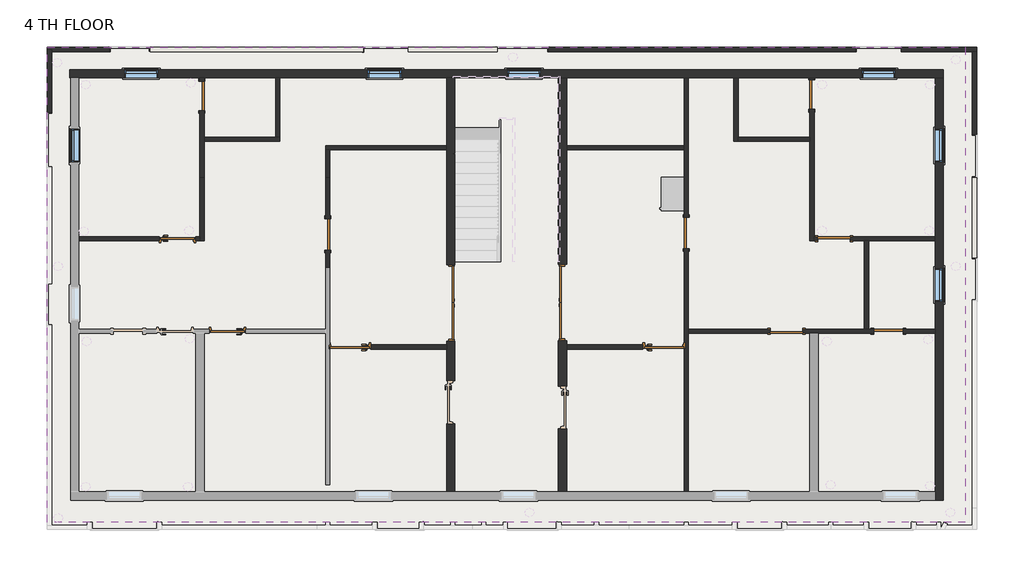
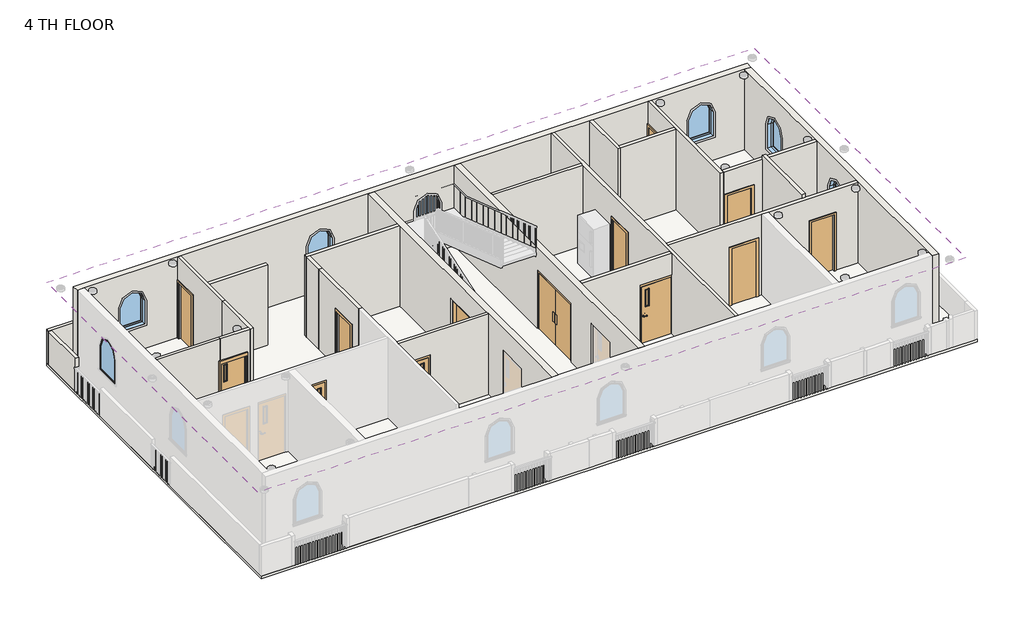
# One storey, part 2 of 7: 32 walls, 13 doors, 7 windows, 1 covering, 1 slab.
# Revit data of these elements (continued)
# Elements 6, 7 (IfcDoor, "Door-Passage-Single-Vision_Lite : 3'X7'") (continued)
#   Swing Angle = 90.00°
#   Rough Width = 3' - 4"
#   Rough Height = 7' - 4"
#   Masonry Inset = 0' - 1"
#   MFOpeningWidth = 0' - 4"
#   MFOpeningHeight = 0' - 4"
#   Inset Calculate = 0' - 4"
#   Masonry Frame = yes
#   Dry Wall Frame = no
#   Phase Created = New Construction
#   Materials on its faces: "Metal - Paint Finish - Grey", "Aluminum", "Wood - Birch", "Glass"
# Elements 8, 9 (IfcDoor, "Single-Flush : 2'10\" x 7'")
#   Phase Created = New Construction
#   Materials on its faces: "Door - Frame", "Door - Panel"
# Elements 10, 11 (IfcDoor, "Single-Flush : 2'11\"x 7'")
#   Phase Created = New Construction
#   Materials on its faces: "Door - Frame", "Door - Panel"
# Elements 12, 13, 14 (IfcDoor, "Single-Flush : 2'8\"x 7'")
#   Phase Created = New Construction
#   Materials on its faces: "Door - Frame", "Door - Panel"
# Element 15 (IfcSlab, "LW Concrete on Metal Deck")
#   Height Offset From Level = 0' - 0"
#   Phase Created = New Construction
#   Materials on its faces: "Metal Deck", "Concrete, Lightweight"
# Elements 16, 17, 18, 19, 20, 21, 22, 23, 24, 25, 26, 27, 28, 29, 31, 32, 33 (IfcWall, "Generic - 4.5\"")
#   Top Offset = -0' - 6"
#   Base Offset = 0' - 0"
#   wall height = 10' - 0"
#   Phase Created = New Construction
#   Base Constraint = 4 TH FLOOR
#   Top Constraint = 5TH FLOOR
#   Materials on its faces: "Default Wall"
# Elements 30, 40 (IfcWall, "Generic - 4.5\"")
#   Top Offset = -6' - 0"
#   Base Offset = 0' - 0"
#   wall height = 4' - 6"
#   Phase Created = New Construction
#   Base Constraint = 4 TH FLOOR
#   Top Constraint = 5TH FLOOR
#   Materials on its faces: "Default Wall"
# Element 34 (IfcWall, "Generic - 4.5\"")
#   Top Offset = -6' - 4.43284"
#   Base Offset = 0' - 0"
#   wall height = 4' - 1.56716"
#   Phase Created = New Construction
#   Base Constraint = 4 TH FLOOR
#   Top Constraint = 5TH FLOOR
#   Materials on its faces: "Default Wall"
# Element 35 (IfcWall, "Generic - 4.5\"")
#   Top Offset = -6' - 3.86561"
#   Base Offset = 0' - 0"
#   wall height = 4' - 2.13439"
#   Phase Created = New Construction
#   Base Constraint = 4 TH FLOOR
#   Top Constraint = 5TH FLOOR
#   Materials on its faces: "Default Wall"
# Element 36 (IfcWall, "Generic - 4.5\"")
#   Top Offset = -6' - 11.32684"
#   Base Offset = 0' - 0"
#   wall height = 3' - 6.67316"
#   Phase Created = New Construction
#   Base Constraint = 4 TH FLOOR
#   Top Constraint = 5TH FLOOR
#   Materials on its faces: "Default Wall"
# Element 37 (IfcWall, "Generic - 4.5\"")
#   Top Offset = -6' - 6.91444"
#   Base Offset = 0' - 0"
#   wall height = 3' - 11.08556"
#   Phase Created = New Construction
#   Base Constraint = 4 TH FLOOR
#   Top Constraint = 5TH FLOOR
#   Materials on its faces: "Default Wall"
# Element 38 (IfcWall, "Generic - 4.5\"")
#   Top Offset = -6' - 3.83516"
#   Base Offset = 0' - 0"
#   wall height = 4' - 2.16484"
#   Phase Created = New Construction
#   Base Constraint = 4 TH FLOOR
#   Top Constraint = 5TH FLOOR
#   Materials on its faces: "Default Wall"
# Element 39 (IfcWall, "Generic - 4.5\"")
#   Top Offset = -6' - 0.2303"
#   Base Offset = 0' - 0"
#   wall height = 4' - 5.7697"
#   Phase Created = New Construction
#   Base Constraint = 4 TH FLOOR
#   Top Constraint = 5TH FLOOR
#   Materials on its faces: "Default Wall"
# Element 41 (IfcWall, "Generic - 4.5\"")
#   Top Offset = -6' - 7.02989"
#   Base Offset = 0' - 0"
#   wall height = 3' - 10.97011"
#   Phase Created = New Construction
#   Base Constraint = 4 TH FLOOR
#   Top Constraint = 5TH FLOOR
#   Materials on its faces: "Default Wall"
# Elements 42, 43, 44, 45 (IfcWall, "Generic - 9\"")
#   Top Offset = -0' - 6"
#   Base Offset = 0' - 0"
#   wall height = 10' - 0"
#   Phase Created = New Construction
#   Base Constraint = 4 TH FLOOR
#   Top Constraint = 5TH FLOOR
#   Materials on its faces: "Concrete Masonry Units"
# Elements 46, 47 (IfcWall, "Interior - 5\" Partition (2-hr)")
#   Top Offset = 0' - 0"
#   Base Offset = 0' - 0"
#   wall height = 10' - 6"
#   Phase Created = New Construction
#   Base Constraint = 4 TH FLOOR
#   Top Constraint = 5TH FLOOR
#   Materials on its faces: "Default Wall", "Gypsum Wall Board"
# Element 48 (IfcWindow, "Window-Fixed-Round-Top : 3' x 4'")
#   Mark = "176"
#   Window Inset = 0' - 0"
#   Interior Wall Closure = 0' - 2 1/4"
#   Frame Extension = 0' - 0 1/4"
#   Exterior Wall Closure = 0' - 1 1/4"
#   Interior Trim Visibility = yes
#   Exterior Trim Visibility = yes
#   Phase Created = New Construction
#   Materials on its faces: "Wood - Stained", "Clad - White", "Glass"
# Element 49 (IfcWindow, "Window-Fixed-Round-Top : 3' x 4'")
#   Mark = "177"
#   Window Inset = 0' - 0"
#   Interior Wall Closure = 0' - 2 1/4"
#   Frame Extension = 0' - 0 1/4"
#   Exterior Wall Closure = 0' - 1 1/4"
#   Interior Trim Visibility = yes
#   Exterior Trim Visibility = yes
#   Phase Created = New Construction
#   Materials on its faces: "Wood - Stained", "Clad - White", "Glass"
# Element 50 (IfcWindow, "Window-Fixed-Round-Top : 3' x 4'")
#   Mark = "178"
#   Window Inset = 0' - 0"
#   Interior Wall Closure = 0' - 2 1/4"
#   Frame Extension = 0' - 0 1/4"
#   Exterior Wall Closure = 0' - 1 1/4"
#   Interior Trim Visibility = yes
#   Exterior Trim Visibility = yes
#   Phase Created = New Construction
#   Materials on its faces: "Wood - Stained", "Clad - White", "Glass"
# Element 51 (IfcWindow, "Window-Fixed-Round-Top : 3' x 4'")
#   Mark = "179"
#   Window Inset = 0' - 0"
#   Interior Wall Closure = 0' - 2 1/4"
#   Frame Extension = 0' - 0 1/4"
#   Exterior Wall Closure = 0' - 1 1/4"
#   Interior Trim Visibility = yes
#   Exterior Trim Visibility = yes
#   Phase Created = New Construction
#   Materials on its faces: "Wood - Stained", "Clad - White", "Glass"
# Element 52 (IfcWindow, "Window-Fixed-Round-Top : 3' x 4'")
#   Mark = "180"
#   Window Inset = 0' - 0"
#   Interior Wall Closure = 0' - 2 1/4"
#   Frame Extension = 0' - 0 1/4"
#   Exterior Wall Closure = 0' - 1 1/4"
#   Interior Trim Visibility = yes
#   Exterior Trim Visibility = yes
#   Phase Created = New Construction
#   Materials on its faces: "Wood - Stained", "Clad - White", "Glass"
# Element 53 (IfcWindow, "Window-Fixed-Round-Top : 3' x 4'")
#   Mark = "181"
#   Window Inset = 0' - 0"
#   Interior Wall Closure = 0' - 2 1/4"
#   Frame Extension = 0' - 0 1/4"
#   Exterior Wall Closure = 0' - 1 1/4"
#   Interior Trim Visibility = yes
#   Exterior Trim Visibility = yes
#   Phase Created = New Construction
#   Materials on its faces: "Wood - Stained", "Clad - White", "Glass"
# Element 54 (IfcWindow, "Window-Fixed-Round-Top : 3' x 4'")
#   Mark = "182"
#   Window Inset = 0' - 0"
#   Interior Wall Closure = 0' - 2 1/4"
#   Frame Extension = 0' - 0 1/4"
#   Exterior Wall Closure = 0' - 1 1/4"
#   Interior Trim Visibility = yes
#   Exterior Trim Visibility = yes
#   Phase Created = New Construction
#   Materials on its faces: "Wood - Stained", "Clad - White", "Glass"
# Materials
#   "Default": colour RGB 127 127 127, transparency 0, Cost = 0
#   "Acoustic Ceiling Tile 24 x 48": class "Generic", colour RGB 229 229 229, transparency 0, Description = "Acoustic Ceiling Tile 24 x 48", Cost = 0
#   "Metal - Paint Finish - Brindle": class "Paint", colour RGB 164 133 98, transparency 0, Cost = 0
#   "Metal - Paint Finish - Grey": class "Paint", colour RGB 104 104 104, transparency 0, Cost = 0
#   "Aluminium": class "Metal", colour RGB 244 244 244, transparency 0, Description = "Aluminum 6061", Cost = 0
#   "Wood - Birch": class "Wood", colour RGB 166 116 52, transparency 0, Cost = 0
#   "Glass": class "Glass", colour RGB 0 128 192, transparency 0.75, Description = "Soda Lime Glass", Cost = 0
#   "Aluminum": class "Metal", colour RGB 247 247 247, transparency 0, Description = "Aluminum 6061", Cost = 0
#   "Door - Panel": class "Wood", colour RGB 210 159 95, transparency 0, Cost = 0
#   "Door - Frame": colour RGB 118 70 51, transparency 0, Cost = 0
#   "Concrete, Lightweight": class "Concrete", colour RGB 142 141 140, transparency 0, Description = "Lightweight concrete", Cost = 0
#   "Metal Deck": class "Metal", colour RGB 199 199 199, transparency 0, Description = "Steel, mill finish", Cost = 0
#   "Concrete Masonry Units": class "Masonry", colour RGB 227 227 227, transparency 0, Description = "Concrete masonry units", Cost = 0
#   "Gypsum Wall Board": class "Generic", colour RGB 127 127 127, transparency 0, Description = "Gypsum Wall Board", Cost = 0
#   "Metal Stud Layer": class "Metal", colour RGB 199 199 199, transparency 0, Description = "Light gauge steel framing, thermal air layer", Cost = 0
#   "Wood - Stained": class "Wood", colour RGB 224 178 126, transparency 0, Cost = 0
#   "Clad - White": class "Wood", colour RGB 242 242 238, transparency 0, Cost = 0
#   "Default Wall": colour RGB 128 128 128, transparency 0, Cost = 0
